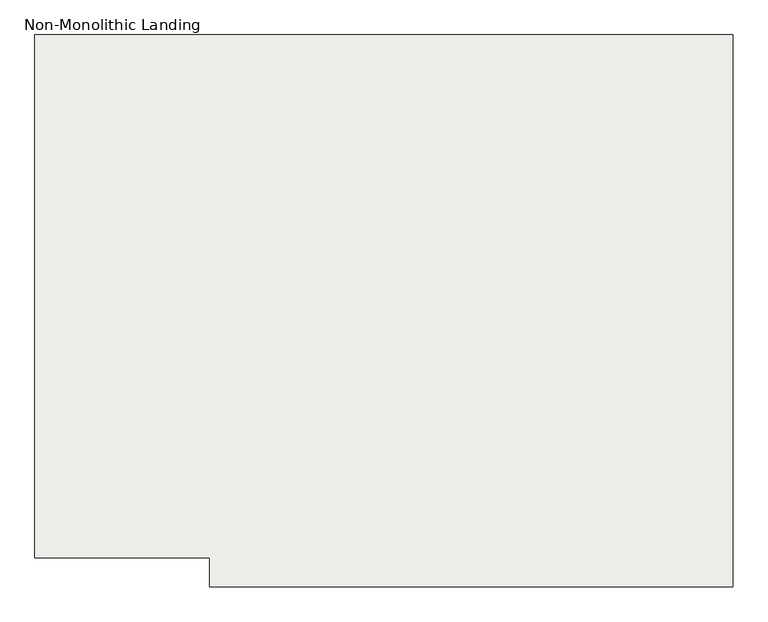
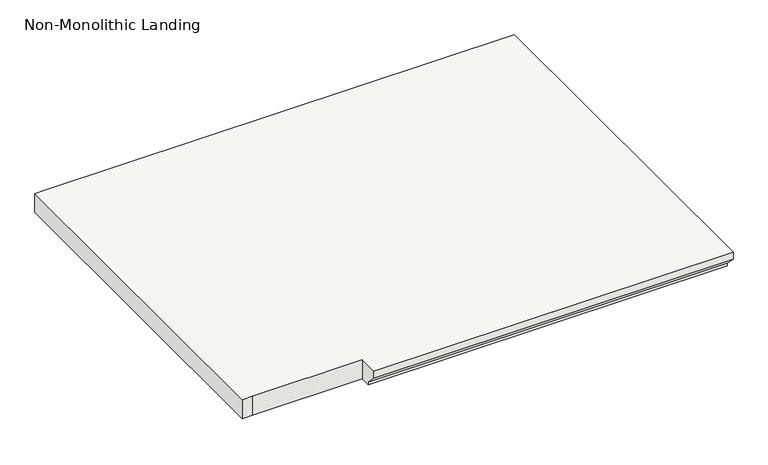
"""IFC4 building model written with IfcOpenShell, lengths in millimetres: slab geometry, Non-Monolithic Landing."""

from ifc_helpers import new_model, si_unit, origin, place, context, project, spatial, faceted_brep, source, transform, mapped, element, save


def non_monolithic_landing_614a383d(model_context):
    return source(origin(), model_context, "Body", "Brep", [
        faceted_brep([(9871.2423568, -8140.7746824, 2098.5078947), (9871.2423568, -8140.7746824, 2117.5578947), (8956.8423568, -8140.7746824, 2117.5578947), (8956.8423568, -8140.7746824, 2098.5078947), (9871.2423568, -8115.3746824, 2073.1078947), (8956.8423568, -8115.3746824, 2073.1078947), (9871.2423568, -7175.5746824, 2117.5578947), (8676.6463344, -7175.5746824, 2117.5578947), (8651.2463344, -7175.5746824, 2117.5578947), (8651.2463344, -8089.9746824, 2117.5578947), (8676.6463344, -8089.9746824, 2117.5578947), (8956.8423568, -8089.9746824, 2117.5578947), (9871.2423568, -8115.3746824, 2066.7578947), (8956.8423568, -8115.3746824, 2066.7578947), (8956.8423568, -8089.9746824, 2066.7578947), (8676.6463344, -8089.9746824, 2066.7578947), (8651.2463344, -8089.9746824, 2066.7578947), (8651.2463344, -7175.5746824, 2066.7578947), (8676.6463344, -7175.5746824, 2066.7578947), (9871.2423568, -7175.5746824, 2066.7578947)], [[[0, 1, 2, 3]], [[4, 0, 3, 5]], [[6, 7, 8, 9, 10, 11, 2, 1]], [[12, 13, 14, 15, 16, 17, 18, 19]], [[13, 12, 4, 5]], [[6, 1, 0, 4, 12, 19]], [[7, 6, 19, 18]], [[8, 7, 18, 17]], [[9, 8, 17, 16]], [[10, 9, 16, 15]], [[11, 10, 15, 14]], [[2, 11, 14, 13, 5, 3]]]),
    ])


if __name__ == "__main__":
    model = new_model("IFC4")
    model_context = context("Model", 3, world=origin())
    ifc_project = project(units=[si_unit("LENGTHUNIT", "METRE", prefix="MILLI")], contexts=[model_context])
    site = spatial("IfcSite", under=ifc_project)
    building = spatial("IfcBuilding", under=site)
    placement = place(None, origin())
    non_monolithic_landing_shape = non_monolithic_landing_614a383d(model_context)
    element("IfcSlab", 1, ObjectType="Non-Monolithic Landing", at=placement, inside=building, context=model_context, shape_type="MappedRepresentation", body=[
        mapped(non_monolithic_landing_shape, transform((0.0, 0.0, 0.0), x_axis=(1.0, 0.0, 0.0), y_axis=(0.0, 1.0, 0.0), z_axis=(0.0, 0.0, 1.0))),
    ])
    save(model, "model.ifc")

# Revit data of these elements
# Element 1 (IfcSlab, "Non-Monolithic Landing")
#   Materials on its faces: "MARBLE STAIRS 6\""
# Materials
#   "MARBLE STAIRS 6\"": class "Generic", colour RGB 120 120 120, transparency 0, Cost = 0
